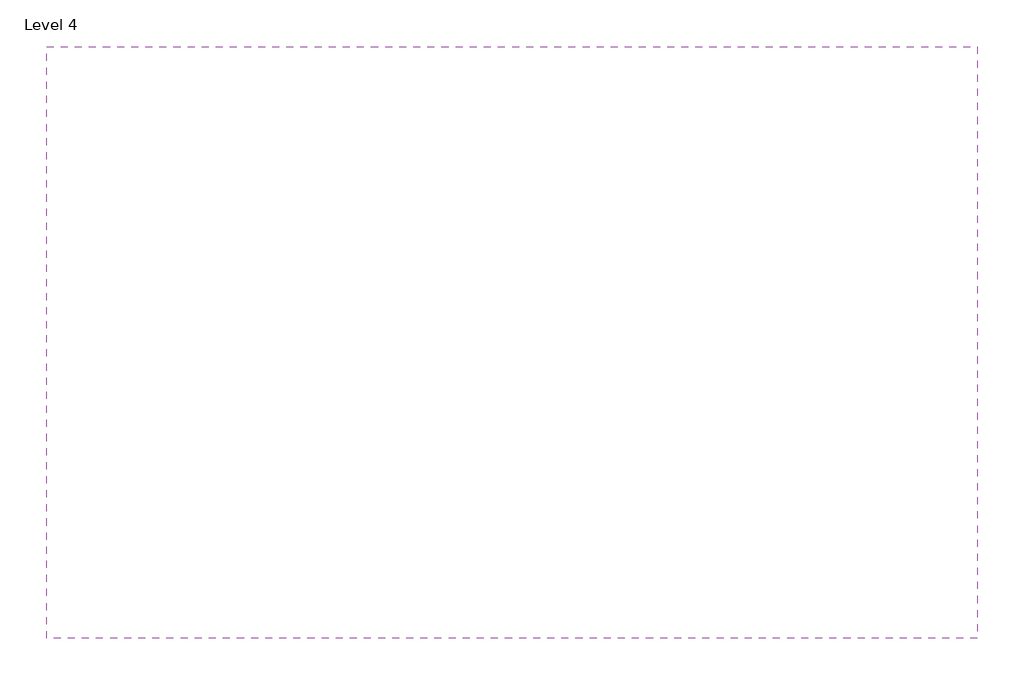
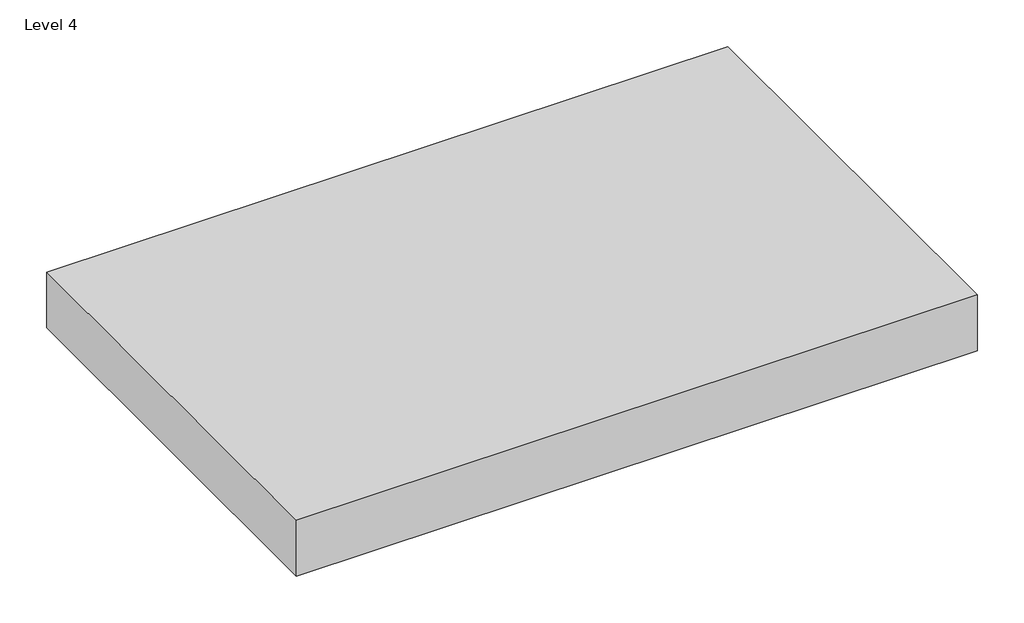
# One storey: 1 proxy.
"""IFC4 building model written with IfcOpenShell, lengths in millimetres."""

from ifc_helpers import new_model, si_unit, origin, place, context, project, spatial, transform, mapped, element, save
from components import generic_models_6_generic_models_6_f9bdd1e7

model = new_model("IFC4")

# Units and contexts
model_context = context("Model", 3, world=origin())
ifc_project = project(units=[si_unit("LENGTHUNIT", "METRE", prefix="MILLI")], contexts=[model_context])

# Site, building, storey
site = spatial("IfcSite", under=ifc_project)
building = spatial("IfcBuilding", under=site)
storey = spatial("IfcBuildingStorey", under=building, Name="Level 4", Elevation=9144.0)

# Proxy
placement = place(None, origin())
generic_models_6_generic_models_6_shape = generic_models_6_generic_models_6_f9bdd1e7(model_context)
element("IfcBuildingElementProxy", 1, Name="Generic Models 6 : Generic Models 6", ObjectType="Generic Models 6 : Generic Models 6", at=placement, inside=storey, context=model_context, shape_type="MappedRepresentation", body=[
    mapped(generic_models_6_generic_models_6_shape, transform((0.0, 0.0, 0.0), x_axis=(1.0, 0.0, 0.0), y_axis=(0.0, 1.0, 0.0), z_axis=(0.0, 0.0, 1.0))),
])

save(model, "model.ifc")

# Revit data of these elements
# Element 1 (IfcBuildingElementProxy, "Generic Models 6 : Generic Models 6")
#   Phase Created = New Construction
